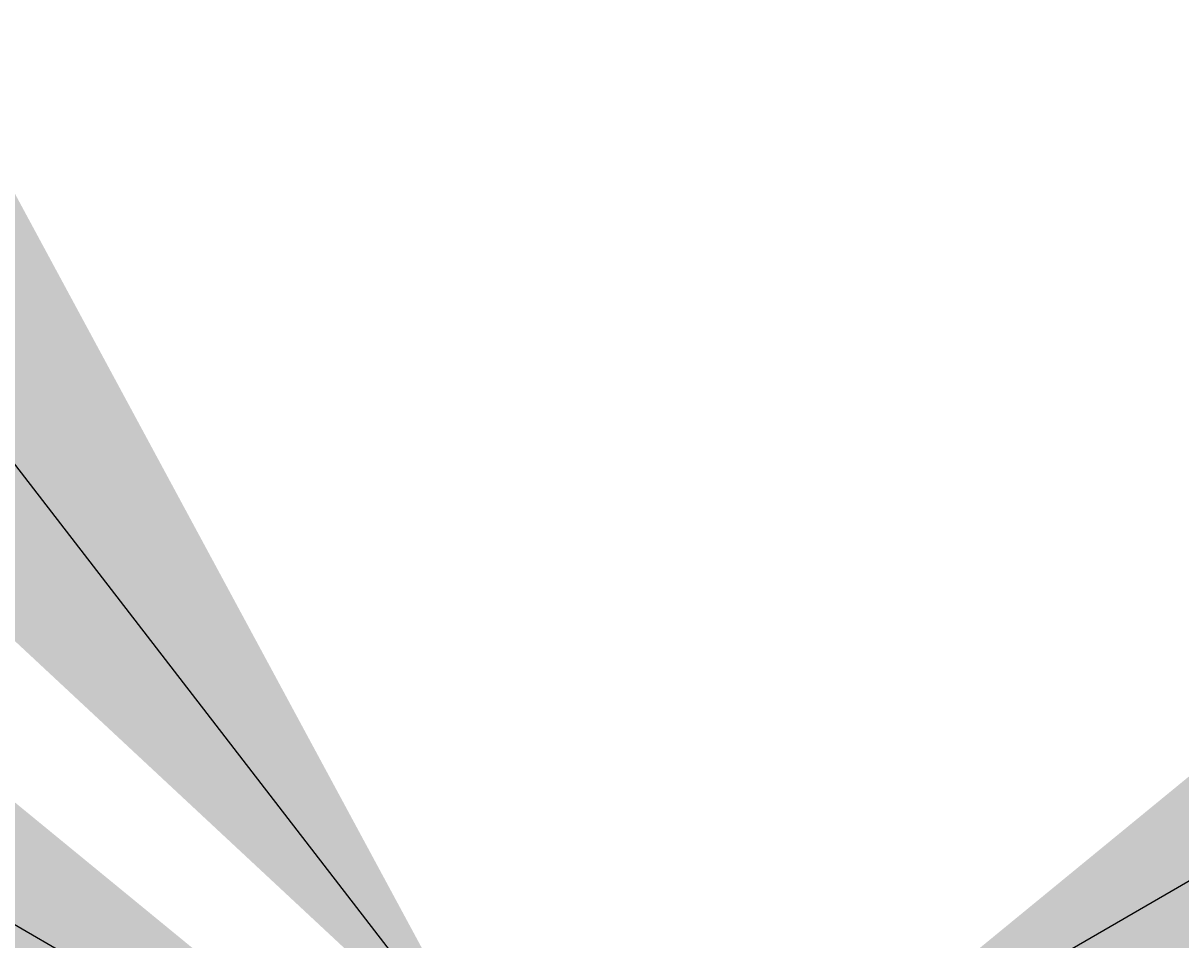
# Model space of a CAD drawing. Units: inches. Extents: x -9413 to 9703, y -9719 to 9096.
# Tile 1 of 1: x -249.7 to 493.3, y 276.8 to 864.8. Entities that reach past the tile are written whole.
import ezdxf
from ezdxf import colors
from ezdxf.entities.mleader import LeaderData, LeaderLine
from ezdxf.math import Vec2, Vec3

# ---------------------------------------------------------------- set-up
doc = ezdxf.new("R2010")
doc.units = ezdxf.units.IN
doc.header["$MEASUREMENT"] = 0
doc.layers.add('M-ANNO-TEXT', color=7, linetype='Continuous', lineweight=18)
doc.styles.get("Standard").update_dxf_attribs({"font": 'arial.ttf'})

msp = doc.modelspace()

# ---------------------------------------------------------------- leaders
at = {"layer": 'M-ANNO-TEXT'}
ml = msp.add_multileader_mtext('Standard', dxfattribs=at)
ml.set_content('steam drum', color=256)
ml.set_leader_properties()
ml.build(insert=Vec2(0, 0))
ml.multileader.update_dxf_attribs({"dogleg_length": 0.36, "arrow_head_size": 10000, "scale": 10})
ctx = ml.context
ctx.base_point, ctx.scale, ctx.char_height, ctx.arrow_head_size, ctx.landing_gap_size, ctx.plane_origin = Vec3(1.078100315116472, 187.1657656808087), 10, 5.4, 10000, 0.9, Vec3(56.53630785249729, 178.1917761520126)
ctx.text_align_type = 2
notes = []
notes.append((ctx, [(0, (1, 1, 0), (49.60206616053652, 187.1657656808087), (-1, 0), 7.616326009130828, [(0, [(56.5363078524973, 178.1917761520126)], 0, [])])]))
ctx.mtext.insert, ctx.mtext.alignment, ctx.mtext.flow_direction = Vec3(41.08574015140569, 189.9099675907678), 3, 5
ml = msp.add_multileader_mtext('Standard', dxfattribs=at)
ml.set_content('Reheater', color=256)
ml.set_leader_properties()
ml.build(insert=Vec2(0, 0))
ml.multileader.update_dxf_attribs({"dogleg_length": 0.36, "arrow_head_size": 10000, "scale": 10})
ctx = ml.context
ctx.base_point, ctx.scale, ctx.char_height, ctx.arrow_head_size, ctx.landing_gap_size, ctx.plane_origin = Vec3(234.1414050860131, 159.7303554673012), 10, 5.4, 10000, 0.9, Vec3(221.1444910066821, 154.3050445940477)
notes.append((ctx, [(0, (1, 1, 0), (230.5414050860131, 159.7303554673012), (1, 0), 3.599999999999999, [(0, [(221.1444910066821, 154.3050445940477)], 0, [])])]))
ctx.mtext.insert, ctx.mtext.flow_direction = Vec3(235.0414050860131, 162.4745573772603), 5
ml = msp.add_multileader_mtext('Standard', dxfattribs=at)
ml.set_content('Boiler', color=256)
ml.set_leader_properties()
ml.build(insert=Vec2(0, 0))
ml.multileader.update_dxf_attribs({"dogleg_length": 0.36, "arrow_head_size": 10000, "scale": 10})
ctx = ml.context
ctx.base_point, ctx.scale, ctx.char_height, ctx.arrow_head_size, ctx.landing_gap_size, ctx.plane_origin = Vec3(31.04430257849453, 103.0991380116177), 10, 5.4, 10000, 0.9, Vec3(69.11352005531556, 99.3051261342938)
ctx.text_align_type = 2
notes.append((ctx, [(0, (1, 1, 0), (62.54209871927075, 103.0991380116177), (-1, 0), 10.86041551321825, [(0, [(69.11352005531556, 99.3051261342938)], 0, [])])]))
ctx.mtext.insert, ctx.mtext.alignment, ctx.mtext.flow_direction = Vec3(50.7816832060525, 105.8433399215768), 3, 5
for ctx, leaders in notes:
    for number, flags, end, landing, length, lines in leaders:
        leader = LeaderData()
        leader.index, (leader.has_last_leader_line, leader.has_dogleg_vector, leader.attachment_direction) = number, flags
        leader.last_leader_point, leader.dogleg_vector, leader.dogleg_length = Vec3(end), Vec3(landing), length
        for number, points, colour, breaks in lines:
            line = LeaderLine()
            line.index, line.vertices, line.color, line.breaks = number, Vec3.list(points), colors.encode_raw_color(colour), breaks
            leader.lines.append(line)
        ctx.leaders.append(leader)

doc.saveas('drawing.dxf')
